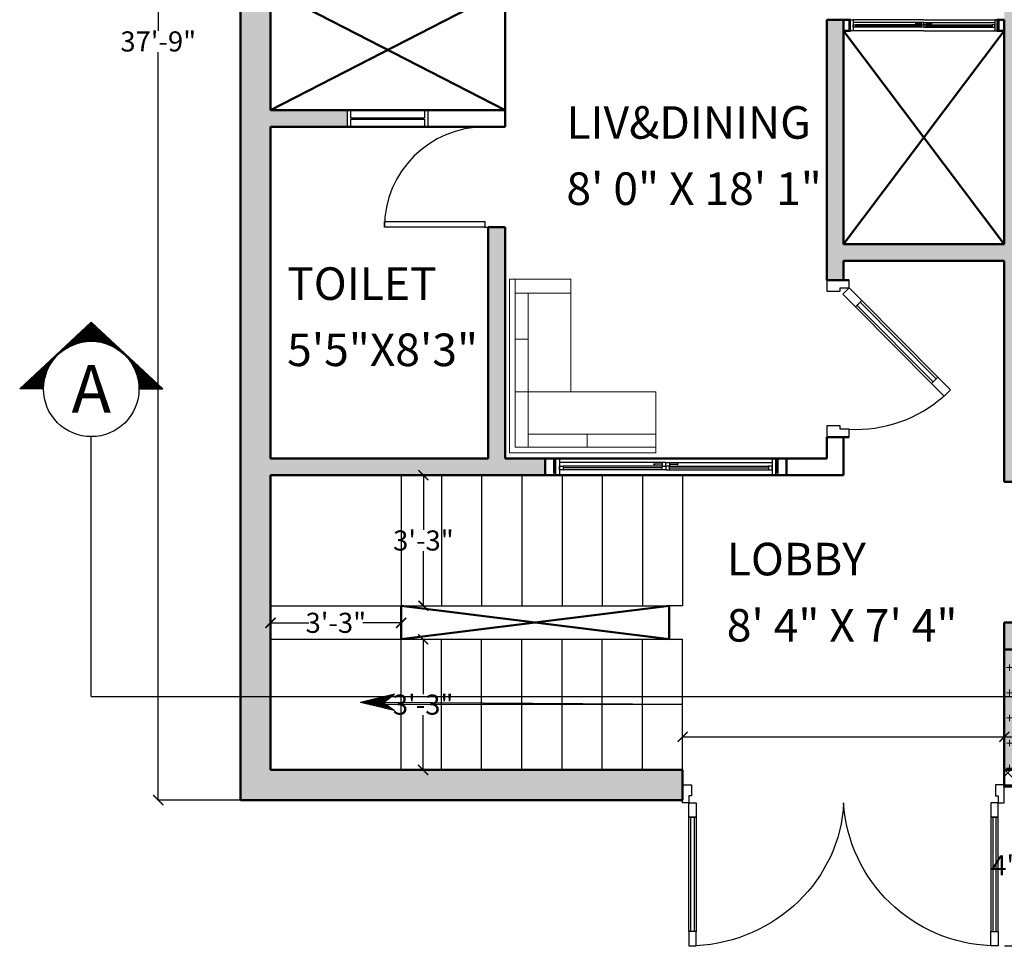
# Model space of a CAD drawing. Units: inches. Extents: x 2278 to 7495, y -71 to 1198.
# Tile 42 of 44: x 6921 to 7215, y 665 to 943. Entities that reach past the tile are written whole.
import ezdxf
from ezdxf.enums import TextEntityAlignment as Align

# ---------------------------------------------------------------- set-up
doc = ezdxf.new("R2010")
doc.units = ezdxf.units.IN
doc.header["$MEASUREMENT"] = 0
for name, color, linetype, lineweight in [('A-ANNO-DIMS', 2, 'Continuous', 18), ('A-ANNO-SYMB', 1, 'Continuous', 25), ('A-AREA-IDEN', 3, 'Continuous', 18), ('A-Door', 3, 'Continuous', 25), ('A-FLOR-PATT', 252, 'Continuous', 13), ('A-FLOR-STRS', 6, 'Continuous', 25), ('A-FURN', 8, 'Continuous', 18), ('A-Glaz', 4, 'Continuous', 25), ('A-Wall', 7, 'Continuous', 50), ('A-WALL-PATT', 8, 'Continuous', 18)]:
    doc.layers.add(name, color=color, linetype=linetype, lineweight=lineweight)
doc.styles.add('KH-TRUC', font='txt', dxfattribs={"height": 200})
doc.styles.get("Standard").update_dxf_attribs({"font": 'arial.ttf'})
doc.dimstyles.get("Standard").update_dxf_attribs({"dimtxt": 6, "dimasz": 3, "dimexe": 0.18, "dimexo": 0.0625, "dimgap": 0.09, "dimtad": 0, "dimtih": 1, "dimtoh": 1, "dimdec": 0, "dimzin": 0, "dimdsep": 46, "dimlunit": 3, "dimtxsty": 'Standard', "dimblk": 'ARCHTICK', "dimcen": 0.09, "dimadec": 0, "dimazin": 0, "dimtfac": 1, "dimtdec": 0, "dimtofl": 0, "dimtmove": 0, "dimatfit": 3, "dimfxl": 1, "dimtolj": 1, "dimtzin": 0, "dimarcsym": 0})

# ---------------------------------------------------------------- blocks, each defined once
blk = doc.blocks.new('*U5')
for p, q in [((0, 0), (0, -6)), ((30, 0), (30, -6))]:
    blk.add_line(p, q)
blk.add_lwpolyline([(0, 0), (0, 30), (1.75, 30), (1.75, 0)], close=True)
blk.add_arc((0, 0), 30, 0, 90)
blk = doc.blocks.new('A$C58286AE3')
for p, q in [((75, 820), (35, 820)), ((35, 820), (35, 180)), ((65, 820), (45, 820)), ((75, 180), (75, 820)), ((75, 180), (35, 180)), ((35, 180), (75, 180)), ((45, 180), (65, 180))]:
    blk.add_line(p, q)
blk.add_lwpolyline([(1725, 180), (1725, 820), (1765, 820), (1765, 180)], close=True)
blk.add_arc((1756.5, 42.1), 858.5, 92.1038, 176.1334)
blk.add_ellipse((70, 105), major_axis=(-772.1, 325.5), ratio=0.94084, start_param=-2.726592, end_param=-1.199193)
at = {"layer": 'A-Door'}
for p, q in [((35, 820), (35, 900)), ((35, 900), (75, 900)), ((75, 900), (75, 820)), ((75, 820), (35, 820)), ((35, 180), (35, 100)), ((75, 100), (75, 180)), ((35, 100), (0, 100)), ((0, 100), (0, 0)), ((35, 60), (35, 100)), ((35, 100), (75, 100)), ((50, 60), (35, 60)), ((50, 50), (50, 60)), ((50, 0), (50, 50)), ((0, 0), (50, 0))]:
    blk.add_line(p, q, dxfattribs=at)
for points in [[(1725, 900), (1725, 820), (1765, 820), (1765, 900)], [(1725, 100), (1725, 180), (1765, 180), (1765, 100)], [(1765, 100), (1800, 100), (1800, 0), (1750, 0), (1750, 50), (1750, 60), (1765, 60)]]:
    blk.add_lwpolyline(points, close=True, dxfattribs=at)
at = {"layer": 'A-Glaz'}
for p, q in [((45, 820), (45, 180)), ((65, 180), (65, 820))]:
    blk.add_line(p, q, dxfattribs=at)
blk.add_lwpolyline([(1735, 180), (1735, 820), (1755, 820), (1755, 180)], close=True, dxfattribs=at)
blk = doc.blocks.new('A$C1DF4181C')
blk.add_lwpolyline([(120, 128), (460.7, 466.1), (432.5, 494.5), (91.8, 156.4)], close=True)
blk.add_arc((72.4, 128.7), 593.3, 357.2313, 41.4937)
at = {"layer": 'A-Door'}
for points in [[(517.5, 522.4), (460.7, 466.1), (432.5, 494.5), (489.3, 550.8)], [(63.2, 71.6), (120, 128), (91.8, 156.4), (35, 100)], [(35, 100), (0, 100), (0, 0), (50, 0), (50, 50), (50, 60), (35, 60)], [(665, 100), (665, 60), (650, 60), (650, 50), (650, 0), (700, 0), (700, 100)]]:
    blk.add_lwpolyline(points, close=True, dxfattribs=at)
at = {"layer": 'A-Glaz'}
blk.add_lwpolyline([(112.9, 135.1), (453.6, 473.2), (439.5, 487.4), (98.8, 149.3)], close=True, dxfattribs=at)
at = {"layer": 'A-Wall'}
for p, q in [((0, 0), (0, 100)), ((0, 100), (0, 0)), ((700, 0), (700, 100)), ((700, 0), (700, 100))]:
    blk.add_line(p, q, dxfattribs=at)
blk = doc.blocks.new('_ArchTick')
at = {"color": 0, "linetype": 'ByBlock', "const_width": 0.15}
blk.add_lwpolyline([(-0.5, -0.5), (0.5, 0.5)], dxfattribs=at)
blk = doc.blocks.new('*D24')
at = {"layer": 'A-ANNO-DIMS', "color": 0, "lineweight": -2, "transparency": 16777216}
for p, q in [((7040.89, 807.47), (7041.94, 807.47)), ((7041.76, 807.47), (7041.76, 791.12)), ((7041.76, 768.47), (7041.76, 784.81)), ((7040.89, 768.47), (7041.94, 768.47))]:
    blk.add_line(p, q, dxfattribs=at)
at = {"layer": 'Defpoints', "color": 0, "transparency": 16777216}
for p in [(7040.83, 807.47), (7040.83, 768.47), (7041.76, 768.47)]:
    blk.add_point(p, dxfattribs=at)
at = {"layer": 'A-ANNO-DIMS', "color": 0, "lineweight": -2, "transparency": 16777216, "xscale": 3, "yscale": 3, "zscale": 3}
for p, rotation in [((7041.76, 807.47), 90), ((7041.76, 768.47), 270)]:
    blk.add_blockref('_ArchTick', p, dxfattribs=dict(at, rotation=rotation))
at = {"layer": 'A-ANNO-DIMS', "color": 0, "transparency": 16777216, "insert": (7041.76, 787.97), "char_height": 6, "attachment_point": 5}
blk.add_mtext('\\A1;3\'-3"', dxfattribs=at)
blk = doc.blocks.new('*D25')
at = {"layer": 'A-ANNO-DIMS', "color": 0, "lineweight": -2, "transparency": 16777216}
for p, q in [((6996.12, 763.4), (6996.12, 763.21)), ((6996.12, 763.39), (7007.55, 763.39)), ((7035.12, 763.39), (7023.68, 763.39)), ((7035.12, 763.4), (7035.12, 763.21))]:
    blk.add_line(p, q, dxfattribs=at)
at = {"layer": 'Defpoints', "color": 0, "transparency": 16777216}
for p in [(6996.12, 763.47), (7035.12, 763.47), (7035.12, 763.39)]:
    blk.add_point(p, dxfattribs=at)
at = {"layer": 'A-ANNO-DIMS', "color": 0, "lineweight": -2, "transparency": 16777216, "xscale": 3, "yscale": 3, "zscale": 3, "rotation": 180}
blk.add_blockref('_ArchTick', (6996.12, 763.39), dxfattribs=at)
at = {"layer": 'A-ANNO-DIMS', "color": 0, "lineweight": -2, "transparency": 16777216, "xscale": 3, "yscale": 3, "zscale": 3}
blk.add_blockref('_ArchTick', (7035.12, 763.39), dxfattribs=at)
at = {"layer": 'A-ANNO-DIMS', "color": 0, "transparency": 16777216, "insert": (7015.62, 763.39), "char_height": 6, "attachment_point": 5}
blk.add_mtext('\\A1;3\'-3"', dxfattribs=at)
blk = doc.blocks.new('*D26')
at = {"layer": 'A-ANNO-DIMS', "color": 0, "lineweight": -2, "transparency": 16777216}
for p, q in [((7040.86, 758.47), (7041.85, 758.47)), ((7041.67, 758.47), (7041.67, 742.12)), ((7041.67, 719.47), (7041.67, 735.81)), ((7040.86, 719.47), (7041.85, 719.47))]:
    blk.add_line(p, q, dxfattribs=at)
at = {"layer": 'Defpoints', "color": 0, "transparency": 16777216}
for p in [(7040.8, 758.47), (7040.8, 719.47), (7041.67, 719.47)]:
    blk.add_point(p, dxfattribs=at)
at = {"layer": 'A-ANNO-DIMS', "color": 0, "lineweight": -2, "transparency": 16777216, "xscale": 3, "yscale": 3, "zscale": 3}
for p, rotation in [((7041.67, 758.47), 90), ((7041.67, 719.47), 270)]:
    blk.add_blockref('_ArchTick', p, dxfattribs=dict(at, rotation=rotation))
at = {"layer": 'A-ANNO-DIMS', "color": 0, "transparency": 16777216, "insert": (7041.67, 738.97), "char_height": 6, "attachment_point": 5}
blk.add_mtext('\\A1;3\'-3"', dxfattribs=at)
blk = doc.blocks.new('*D27')
at = {"layer": 'A-ANNO-DIMS', "color": 0, "lineweight": -2, "transparency": 16777216}
for p, q in [((6987.05, 1163.47), (6962.44, 1163.47)), ((6962.62, 1163.47), (6962.62, 940.12)), ((6962.62, 710.47), (6962.62, 933.81)), ((6987.05, 710.47), (6962.44, 710.47))]:
    blk.add_line(p, q, dxfattribs=at)
at = {"layer": 'Defpoints', "color": 0, "transparency": 16777216}
for p in [(6987.12, 1163.47), (6962.62, 710.47), (6987.12, 710.47)]:
    blk.add_point(p, dxfattribs=at)
at = {"layer": 'A-ANNO-DIMS', "color": 0, "lineweight": -2, "transparency": 16777216, "xscale": 3, "yscale": 3, "zscale": 3}
for p, rotation in [((6962.62, 1163.47), 90), ((6962.62, 710.47), 270)]:
    blk.add_blockref('_ArchTick', p, dxfattribs=dict(at, rotation=rotation))
at = {"layer": 'A-ANNO-DIMS', "color": 0, "transparency": 16777216, "insert": (6962.62, 936.97), "char_height": 6, "attachment_point": 5}
blk.add_mtext('\\A1;37\'-9"', dxfattribs=at)
blk = doc.blocks.new('*X31')
at = {"color": 0}
for p, q in [((19.68, 20.47), (19.71, 20.51)), ((19.68, 20.38), (19.76, 20.46)), ((19.68, 20.29), (19.8, 20.42)), ((19.68, 20.21), (19.84, 20.37)), ((19.68, 20.12), (19.88, 20.33)), ((19.68, 20.03), (19.93, 20.28)), ((19.68, 19.94), (19.97, 20.23)), ((19.68, 19.85), (20.01, 20.19)), ((19.68, 19.76), (20.05, 20.14)), ((19.68, 19.68), (20.1, 20.1)), ((19.68, 19.59), (20.14, 20.05)), ((19.68, 19.5), (20.18, 20.01)), ((19.68, 19.41), (20.22, 19.96)), ((19.68, 19.32), (20.27, 19.91)), ((19.68, 19.23), (20.31, 19.87)), ((19.68, 19.15), (20.35, 19.82)), ((19.68, 19.06), (20.4, 19.78)), ((19.68, 18.97), (20.44, 19.73)), ((19.68, 18.88), (20.48, 19.69)), ((19.68, 18.79), (20.52, 19.64)), ((19.68, 18.7), (20.57, 19.59)), ((19.68, 18.62), (20.61, 19.55)), ((19.68, 18.53), (20.65, 19.5)), ((19.68, 18.44), (20.69, 19.46)), ((19.68, 18.35), (20.74, 19.41)), ((19.68, 18.26), (20.78, 19.37)), ((19.68, 18.17), (20.82, 19.32)), ((19.68, 18.08), (20.86, 19.27)), ((19.73, 18.05), (20.91, 19.23)), ((19.81, 18.05), (20.95, 19.18)), ((19.9, 18.04), (20.99, 19.14)), ((19.98, 18.04), (21.04, 19.09)), ((20.06, 18.03), (21.08, 19.05)), ((20.15, 18.03), (21.12, 19)), ((20.23, 18.02), (21.16, 18.95)), ((20.31, 18.01), (21.21, 18.91)), ((20.38, 18), (21.25, 18.86)), ((20.46, 17.99), (21.29, 18.82)), ((20.54, 17.97), (21.33, 18.77)), ((20.61, 17.96), (21.38, 18.73)), ((20.68, 17.94), (21.42, 18.68)), ((20.76, 17.93), (21.46, 18.63)), ((20.83, 17.91), (21.5, 18.59)), ((20.9, 17.9), (21.55, 18.54)), ((20.97, 17.88), (21.59, 18.5)), ((21.04, 17.86), (21.63, 18.45)), ((21.11, 17.84), (21.68, 18.41)), ((21.18, 17.82), (21.72, 18.36)), ((21.24, 17.8), (21.76, 18.31)), ((21.31, 17.77), (21.8, 18.27)), ((21.37, 17.75), (21.85, 18.22)), ((21.44, 17.73), (21.89, 18.18)), ((21.5, 17.7), (21.93, 18.13)), ((21.57, 17.68), (21.97, 18.08)), ((21.63, 17.65), (22.02, 18.04)), ((21.69, 17.62), (22.06, 17.99)), ((21.75, 17.6), (22.1, 17.95)), ((21.81, 17.57), (22.14, 17.9)), ((21.87, 17.54), (22.19, 17.86)), ((21.93, 17.51), (22.23, 17.81)), ((21.99, 17.48), (22.27, 17.76)), ((22.05, 17.45), (22.32, 17.72)), ((22.1, 17.42), (22.36, 17.67)), ((22.16, 17.39), (22.4, 17.63)), ((22.22, 17.35), (22.44, 17.58)), ((22.27, 17.32), (22.49, 17.54)), ((22.33, 17.29), (22.53, 17.49)), ((22.38, 17.25), (22.57, 17.44)), ((22.43, 17.22), (22.61, 17.4)), ((22.49, 17.18), (22.66, 17.35)), ((22.54, 17.15), (22.7, 17.31)), ((22.59, 17.11), (22.74, 17.26)), ((22.64, 17.07), (22.78, 17.22)), ((22.69, 17.04), (22.83, 17.17)), ((22.74, 17), (22.87, 17.12)), ((22.79, 16.96), (22.91, 17.08)), ((22.84, 16.92), (22.96, 17.03)), ((22.89, 16.88), (23, 16.99)), ((22.94, 16.84), (23.04, 16.94)), ((22.98, 16.8), (23.08, 16.9)), ((23.03, 16.75), (23.13, 16.85)), ((23.08, 16.71), (23.17, 16.8)), ((23.12, 16.67), (23.21, 16.76)), ((23.17, 16.63), (23.25, 16.71)), ((23.21, 16.58), (23.3, 16.67)), ((23.26, 16.54), (23.34, 16.62)), ((23.3, 16.49), (23.38, 16.58)), ((23.34, 16.45), (23.42, 16.53)), ((23.38, 16.4), (23.47, 16.48)), ((23.43, 16.35), (23.51, 16.44)), ((23.47, 16.31), (23.55, 16.39)), ((23.51, 16.26), (23.6, 16.35)), ((23.55, 16.21), (23.64, 16.3)), ((23.59, 16.16), (23.68, 16.26)), ((23.63, 16.11), (23.72, 16.21)), ((23.66, 16.06), (23.77, 16.16)), ((23.7, 16.01), (23.81, 16.12)), ((23.74, 15.96), (23.85, 16.07)), ((23.78, 15.91), (23.89, 16.03)), ((23.81, 15.86), (23.94, 15.98)), ((23.85, 15.8), (23.98, 15.94)), ((23.88, 15.75), (24.02, 15.89)), ((23.92, 15.7), (24.06, 15.84)), ((23.95, 15.64), (24.11, 15.8)), ((23.98, 15.59), (24.15, 15.75)), ((24.02, 15.53), (24.19, 15.71)), ((24.05, 15.47), (24.24, 15.66)), ((24.08, 15.42), (24.28, 15.62)), ((24.11, 15.36), (24.32, 15.57)), ((24.14, 15.3), (24.36, 15.52)), ((24.17, 15.24), (24.41, 15.48)), ((24.2, 15.18), (24.45, 15.43)), ((24.23, 15.12), (24.49, 15.39)), ((24.25, 15.06), (24.53, 15.34)), ((24.28, 15), (24.58, 15.3)), ((24.31, 14.94), (24.62, 15.25)), ((24.33, 14.87), (24.66, 15.2)), ((24.36, 14.81), (24.7, 15.16)), ((24.38, 14.74), (24.75, 15.11)), ((24.4, 14.68), (24.79, 15.07)), ((24.42, 14.61), (24.83, 15.02)), ((24.45, 14.55), (24.88, 14.98)), ((24.47, 14.48), (24.92, 14.93)), ((24.49, 14.41), (24.96, 14.88)), ((24.51, 14.34), (25, 14.84)), ((24.52, 14.27), (25.05, 14.79)), ((24.54, 14.2), (25.09, 14.75)), ((24.56, 14.13), (25.13, 14.7)), ((24.57, 14.06), (25.17, 14.66)), ((24.59, 13.98), (25.22, 14.61)), ((24.6, 13.91), (25.26, 14.56)), ((24.61, 13.83), (25.3, 14.52)), ((24.63, 13.75), (25.35, 14.47)), ((24.44, 11.54), (26.33, 13.42)), ((24.48, 11.66), (26.28, 13.47)), ((24.51, 11.79), (26.24, 13.51)), ((24.54, 11.9), (26.2, 13.56)), ((24.57, 12.02), (26.16, 13.6)), ((24.59, 12.13), (26.11, 13.65)), ((24.61, 12.24), (26.07, 13.7)), ((24.63, 12.34), (26.03, 13.74)), ((24.64, 13.68), (25.39, 14.43)), ((24.64, 12.44), (25.99, 13.79)), ((24.65, 13.6), (25.43, 14.38)), ((24.65, 13.52), (25.47, 14.34)), ((24.65, 12.54), (25.94, 13.83)), ((24.66, 13.44), (25.52, 14.29)), ((24.66, 12.64), (25.9, 13.88)), ((24.67, 13.35), (25.56, 14.24)), ((24.67, 13.27), (25.6, 14.2)), ((24.67, 13.18), (25.64, 14.15)), ((24.67, 12.92), (25.77, 14.02)), ((24.67, 12.83), (25.81, 13.97)), ((24.67, 12.73), (25.86, 13.92)), ((24.68, 13.1), (25.69, 14.11)), ((24.68, 13.01), (25.73, 14.06)), ((23.72, 10.11), (26.67, 13.06)), ((23.91, 10.38), (26.63, 13.1)), ((24.04, 10.6), (26.58, 13.15)), ((24.14, 10.79), (26.54, 13.19)), ((24.22, 10.96), (26.5, 13.24)), ((24.29, 11.12), (26.45, 13.28)), ((24.35, 11.27), (26.41, 13.33)), ((24.4, 11.41), (26.37, 13.38)), ((19.68, 5.98), (25.68, 11.98)), ((19.68, 5.89), (24.44, 10.65)), ((19.68, 5.8), (23.2, 9.32)), ((19.68, 6.06), (22.61, 9)), ((19.68, 6.15), (22.34, 8.81)), ((19.68, 6.24), (22.12, 8.69)), ((19.68, 6.33), (21.93, 8.58)), ((19.68, 6.42), (21.76, 8.5)), ((19.68, 6.51), (21.6, 8.43)), ((19.68, 6.59), (21.46, 8.37)), ((19.68, 6.68), (21.32, 8.32)), ((19.68, 6.77), (21.19, 8.28)), ((19.68, 6.86), (21.06, 8.24)), ((19.68, 6.95), (20.94, 8.21)), ((19.68, 7.04), (20.82, 8.18)), ((19.68, 7.12), (20.71, 8.15)), ((19.68, 7.21), (20.6, 8.13)), ((19.68, 7.3), (20.49, 8.11)), ((19.68, 7.39), (20.38, 8.1)), ((19.68, 7.48), (20.28, 8.08)), ((19.68, 7.57), (20.18, 8.07)), ((19.68, 7.74), (19.99, 8.06)), ((19.68, 7.66), (20.08, 8.06)), ((19.68, 8.01), (19.71, 8.05)), ((19.68, 7.92), (19.8, 8.05)), ((19.68, 7.83), (19.9, 8.05)), ((19.68, 5.71), (21.96, 8)), ((19.68, 5.62), (20.73, 6.67))]:
    blk.add_line(p, q, dxfattribs=at)
blk = doc.blocks.new('A$C695C76AC')
for p, q in [((5.36, 5), (12.86, 12)), ((20.36, 5), (12.86, 12)), ((7.86, 5), (5.36, 5)), ((17.86, 5), (20.36, 5))]:
    blk.add_line(p, q)
blk.add_circle((12.86, 5), 5)
at = {"rotation": 90}
blk.add_blockref('*X31', (25.9, -14.68), dxfattribs=at)
at = {"style": 'KH-TRUC'}
blk.add_attdef('KH-MC', text='', height=5, dxfattribs=at).set_placement((12.86, 5), align=Align.MIDDLE_CENTER)
blk = doc.blocks.new('*D55')
at = {"layer": 'A-ANNO-DIMS', "color": 0, "lineweight": -2, "transparency": 16777216}
for p, q in [((7119.12, 715.03), (7119.12, 729.55)), ((7119.12, 729.37), (7215.12, 729.37)), ((7215.12, 715.03), (7215.12, 729.55)), ((7215.12, 729.37), (7218.12, 729.37))]:
    blk.add_line(p, q, dxfattribs=at)
at = {"layer": 'Defpoints', "color": 0, "transparency": 16777216}
for p in [(7215.12, 729.37), (7119.12, 714.97), (7215.12, 714.97)]:
    blk.add_point(p, dxfattribs=at)
at = {"layer": 'A-ANNO-DIMS', "color": 0, "lineweight": -2, "transparency": 16777216, "xscale": 3, "yscale": 3, "zscale": 3, "rotation": 180}
blk.add_blockref('_ArchTick', (7119.12, 729.37), dxfattribs=at)
at = {"layer": 'A-ANNO-DIMS', "color": 0, "lineweight": -2, "transparency": 16777216, "xscale": 3, "yscale": 3, "zscale": 3}
blk.add_blockref('_ArchTick', (7215.12, 729.37), dxfattribs=at)
at = {"layer": 'A-ANNO-DIMS', "color": 0, "transparency": 16777216, "insert": (7285.95, 729.37), "char_height": 6, "attachment_point": 5}
blk.add_mtext('\\A1;MAIN ENTRANCE DOOR 8\'-0" TYP.', dxfattribs=at)
blk = doc.blocks.new('*D56')
at = {"layer": 'A-ANNO-DIMS', "color": 0, "lineweight": -2, "transparency": 16777216}
for p, q in [((7215.18, 714.97), (7229.7, 714.97)), ((7229.52, 714.97), (7229.52, 694.12)), ((7229.52, 666.97), (7229.52, 687.81)), ((7215.18, 666.97), (7229.7, 666.97))]:
    blk.add_line(p, q, dxfattribs=at)
at = {"layer": 'Defpoints', "color": 0, "transparency": 16777216}
for p in [(7215.12, 714.97), (7215.12, 666.97), (7229.52, 666.97)]:
    blk.add_point(p, dxfattribs=at)
at = {"layer": 'A-ANNO-DIMS', "color": 0, "lineweight": -2, "transparency": 16777216, "xscale": 3, "yscale": 3, "zscale": 3}
for p, rotation in [((7229.52, 714.97), 90), ((7229.52, 666.97), 270)]:
    blk.add_blockref('_ArchTick', p, dxfattribs=dict(at, rotation=rotation))
at = {"layer": 'A-ANNO-DIMS', "color": 0, "transparency": 16777216, "insert": (7229.52, 690.97), "char_height": 6, "attachment_point": 5}
blk.add_mtext('\\A1;4\'-0" TYP.', dxfattribs=at)

msp = doc.modelspace()

# ---------------------------------------------------------------- hatches: boundary and pattern name
at = {"layer": 'A-FLOR-PATT'}
h = msp.add_hatch(dxfattribs=at)
h.set_pattern_fill('ANSI31', color=256)
h.set_pattern_definition([(45, (4673.24527, 0), (-0.0883883476, 0.0883883476), [])])
h.paths.add_polyline_path([(7029.84, 739.64), (7033.16, 742.09), (7022.93, 739.64), (7033.16, 737.18)])
at = {"layer": 'A-WALL-PATT'}
h = msp.add_hatch(dxfattribs=at)
h.set_pattern_fill('ANSI36', color=256, scale=30)
h.set_pattern_definition([(45, (4673.2453, 0), (1.988738, 7.2920387), [9.375, -1.875, 0, -1.875])])
h.paths.add_polyline_path([(7016.37, 957.47), (6996.12, 957.47), (6996.12, 1029.47), (7025.12, 1029.47), (7025.12, 1034.47), (6996.12, 1034.47), (6996.12, 1154.47), (7013.12, 1154.47), (7013.12, 1163.47), (6987.12, 1163.47), (6987.12, 710.47), (7119.12, 710.47), (7119.12, 719.47), (6996.12, 719.47), (6996.12, 807.47), (7078.12, 807.47), (7078.12, 812.47), (7066.12, 812.47), (7066.12, 881.47), (7061.12, 881.47), (7061.12, 812.47), (6996.12, 812.47), (6996.12, 911.47), (7019.12, 911.47), (7019.12, 916.47), (6996.12, 916.47), (6996.12, 952.47), (7016.37, 952.47)])
h.paths.add_polyline_path([(7125.12, 1163.47), (7085.12, 1163.47), (7085.12, 1154.47), (7102.12, 1154.47), (7102.12, 1034.47), (7102.12, 1029.47), (7107.12, 1029.47), (7107.12, 1154.47), (7125.12, 1154.47)])
h.paths.add_polyline_path([(7232.12, 1163.47), (7197.12, 1163.47), (7197.12, 1154.47), (7215.12, 1154.47), (7215.12, 1034.47), (7149.12, 1034.47), (7149.12, 1029.47), (7215.12, 1029.47), (7215.12, 943.47), (7215.12, 940.13), (7215.12, 876.47), (7167.12, 876.47), (7167.12, 943.47), (7162.12, 943.47), (7162.12, 871.47), (7162.12, 865.74), (7167.12, 865.74), (7167.12, 871.47), (7215.12, 871.47), (7215.12, 805.47), (7220.12, 805.47), (7220.12, 1077.47), (7232.12, 1077.47), (7232.12, 1082.47), (7220.12, 1082.47), (7220.12, 1154.47), (7232.12, 1154.47)])
h.paths.add_polyline_path([(7390.12, 937.97), (7381.12, 937.97), (7381.12, 911.47), (7268.12, 911.47), (7268.12, 906.47), (7381.12, 906.47), (7381.12, 869.47), (7390.12, 869.47)])
h.paths.add_polyline_path([(7390.12, 1163.47), (7363.12, 1163.47), (7363.12, 1154.47), (7381.12, 1154.47), (7381.12, 1041.47), (7268.12, 1041.47), (7268.12, 1036.47), (7381.12, 1036.47), (7381.12, 1009.97), (7390.12, 1009.97)])
h.paths.add_polyline_path([(7291.12, 1163.47), (7256.12, 1163.47), (7256.12, 1154.47), (7268.12, 1154.47), (7268.12, 1082.47), (7262.12, 1082.47), (7262.12, 1077.47), (7273.12, 1077.47), (7273.12, 1154.47), (7291.12, 1154.47)])
h.paths.add_polyline_path([(7390.12, 797.47), (7381.12, 797.47), (7381.12, 760.47), (7336.62, 760.47), (7336.62, 755.47), (7390.12, 755.47)])
h.paths.add_polyline_path([(7264.62, 760.47), (7220.12, 760.47), (7220.12, 763.47), (7215.12, 763.47), (7215.12, 755.47), (7264.62, 755.47)])
h = msp.add_hatch(dxfattribs=at)
h.set_pattern_fill('ANSI37', color=256, scale=30)
h.set_pattern_definition([(45, (4673.2453, 0), (-2.6516504, 2.6516504), []), (135, (4673.2453, 0), (-2.6516504, -2.6516504), [])])
h.paths.add_polyline_path([(7390.12, 755.47), (7381.12, 755.47), (7381.12, 719.47), (7215.12, 719.47), (7215.12, 714.47), (7390.12, 714.47)])
at = {"layer": 'A-WALL-PATT', "transparency": 33554562}
h = msp.add_hatch(color=256, dxfattribs=at)
h.dxf.hatch_style = 1
h.paths.add_polyline_path([(7381.12, 755.47), (7215.12, 755.47), (7215.12, 719.47), (7381.12, 719.47)])
h = msp.add_hatch(dxfattribs=at)
h.set_pattern_fill('CROSS', color=256, scale=15)
h.set_pattern_definition([(0, (4673.2453, 0), (3.75, 3.75), [1.875, -5.625]), (90, (4674.1828, -0.9375), (-3.75, 3.75), [1.875, -5.625])])
h.paths.add_polyline_path([(7381.12, 755.47), (7215.12, 755.47), (7215.12, 719.47), (7381.12, 719.47)])

# ---------------------------------------------------------------- linework, layer by layer
at = {"layer": 'A-ANNO-SYMB'}
for q in [(6942.63, 818.97), (7473.67, 741.41)]:
    msp.add_line((6942.63, 741.41), q, dxfattribs=at)
at = {"layer": 'A-FLOR-STRS'}
for p, q in [((7035.12, 807.47), (7035.12, 768.47)), ((7047.12, 807.47), (7047.12, 768.47)), ((7059.12, 807.47), (7059.12, 768.47)), ((7071.12, 807.47), (7071.12, 768.47)), ((7083.12, 807.47), (7083.12, 768.47)), ((7095.12, 807.47), (7095.12, 768.47)), ((7107.12, 807.47), (7107.12, 768.47)), ((7119.12, 807.47), (7119.12, 768.47)), ((6996.12, 768.47), (7115.12, 768.47)), ((7119.12, 768.47), (7115.12, 768.47)), ((6996.12, 758.47), (7119.12, 758.47)), ((7035.12, 719.47), (7035.12, 758.47)), ((7047.12, 719.47), (7047.12, 758.47)), ((7059.12, 719.47), (7059.12, 758.47)), ((7071.12, 719.47), (7071.12, 758.47)), ((7083.12, 719.47), (7083.12, 758.47)), ((7095.12, 719.47), (7095.12, 758.47)), ((7107.12, 719.47), (7107.12, 758.47)), ((7119.12, 719.47), (7119.12, 758.47)), ((7033.16, 742.09), (7022.93, 739.64)), ((7029.84, 739.64), (7033.16, 742.09)), ((7033.16, 737.18), (7022.93, 739.64)), ((7119.12, 738.97), (7029.84, 739.64)), ((7029.84, 739.64), (7033.16, 737.18)), ((7119.12, 738.97), (7030.58, 738.97))]:
    msp.add_line(p, q, dxfattribs=at)
at = {"layer": 'A-FURN'}
for p, q in [((7067.46, 814.1), (7067.46, 866.04)), ((7085.7, 866.04), (7067.46, 866.04)), ((7069.15, 815.79), (7069.15, 866.04)), ((7085.7, 832.34), (7085.7, 866.04)), ((7085.7, 861.82), (7069.15, 861.82)), ((7073.03, 815.79), (7073.03, 861.82)), ((7073.03, 848.05), (7069.15, 848.05)), ((7111.07, 832.34), (7069.15, 832.34)), ((7111.07, 814.1), (7111.07, 832.34)), ((7073.03, 819.67), (7111.07, 819.67)), ((7090.59, 815.79), (7090.59, 819.67)), ((7111.07, 814.1), (7067.46, 814.1)), ((7069.15, 815.79), (7111.07, 815.79))]:
    msp.add_line(p, q, dxfattribs=at)
at = {"layer": 'A-Glaz'}
for p, q in [((7191.12, 943.47), (7169.97, 943.47)), ((7191.12, 943.47), (7212.26, 943.47)), ((7191.12, 942.66), (7169.97, 942.66)), ((7190.39, 941.94), (7170.69, 941.94)), ((7190.39, 941.58), (7170.69, 941.58)), ((7190.39, 941.22), (7170.69, 941.22)), ((7190.39, 942.3), (7188.84, 942.3)), ((7191.12, 942.66), (7212.26, 942.66)), ((7191.84, 942.3), (7193.39, 942.3)), ((7191.84, 941.94), (7211.54, 941.94)), ((7191.84, 941.58), (7211.54, 941.58)), ((7191.84, 941.22), (7211.54, 941.22)), ((7191.12, 940.13), (7169.97, 940.13)), ((7191.12, 940.13), (7212.26, 940.13)), ((7019.12, 916.47), (7043.12, 916.47)), ((7019.12, 911.47), (7019.12, 916.47)), ((7020.12, 914.17), (7020.12, 916.47)), ((7020.12, 914.17), (7042.12, 914.17)), ((7042.12, 916.47), (7042.12, 914.17)), ((7043.12, 916.47), (7043.12, 911.47)), ((7043.12, 911.47), (7019.12, 911.47)), ((7020.12, 911.47), (7020.12, 913.77)), ((7020.12, 913.77), (7042.12, 913.77)), ((7042.12, 913.77), (7042.12, 911.47)), ((7114.12, 812.47), (7082.39, 812.47)), ((7114.12, 811.26), (7082.39, 811.26)), ((7114.12, 812.47), (7145.84, 812.47)), ((7114.12, 811.26), (7145.84, 811.26)), ((7113.03, 810.18), (7083.48, 810.18)), ((7113.03, 809.64), (7083.48, 809.64)), ((7113.03, 809.09), (7083.48, 809.09)), ((7113.03, 810.72), (7110.7, 810.72)), ((7115.2, 810.72), (7117.53, 810.72)), ((7115.2, 810.18), (7144.75, 810.18)), ((7115.2, 809.64), (7144.75, 809.64)), ((7115.2, 809.09), (7144.75, 809.09)), ((7114.12, 807.47), (7082.39, 807.47)), ((7114.12, 807.47), (7145.84, 807.47))]:
    msp.add_line(p, q, dxfattribs=at)
for points in [[(7169.97, 940.13), (7169.24, 940.13), (7169.24, 943.47), (7169.97, 943.47)], [(7212.26, 940.13), (7212.99, 940.13), (7212.99, 943.47), (7212.26, 943.47)], [(7170.69, 941.22), (7169.97, 941.22), (7169.97, 941.94), (7170.69, 941.94)], [(7188.65, 942.3), (7188.84, 942.41), (7188.84, 942.19)], [(7190.39, 941.94), (7191.12, 941.94), (7191.12, 942.66), (7190.39, 942.66)], [(7191.12, 941.22), (7190.39, 941.22), (7190.39, 941.94), (7191.12, 941.94)], [(7191.84, 941.94), (7191.12, 941.94), (7191.12, 942.66), (7191.84, 942.66)], [(7191.12, 941.22), (7191.84, 941.22), (7191.84, 941.94), (7191.12, 941.94)], [(7193.58, 942.3), (7193.39, 942.41), (7193.39, 942.19)], [(7211.54, 941.22), (7212.26, 941.22), (7212.26, 941.94), (7211.54, 941.94)], [(7082.39, 807.47), (7081.31, 807.47), (7081.31, 812.47), (7082.39, 812.47)], [(7113.03, 810.18), (7114.12, 810.18), (7114.12, 811.26), (7113.03, 811.26)], [(7115.2, 810.18), (7114.12, 810.18), (7114.12, 811.26), (7115.2, 811.26)], [(7145.84, 807.47), (7146.92, 807.47), (7146.92, 812.47), (7145.84, 812.47)], [(7083.48, 809.09), (7082.39, 809.09), (7082.39, 810.18), (7083.48, 810.18)], [(7110.42, 810.72), (7110.7, 810.88), (7110.7, 810.56)], [(7114.12, 809.09), (7113.03, 809.09), (7113.03, 810.18), (7114.12, 810.18)], [(7114.12, 809.09), (7115.2, 809.09), (7115.2, 810.18), (7114.12, 810.18)], [(7117.81, 810.72), (7117.53, 810.88), (7117.53, 810.56)], [(7144.75, 809.09), (7145.84, 809.09), (7145.84, 810.18), (7144.75, 810.18)]]:
    msp.add_lwpolyline(points, close=True, dxfattribs=at)
at = {"layer": 'A-Wall'}
for p, q in [((6987.12, 1163.47), (6987.12, 710.47)), ((7066.12, 1029.47), (7066.12, 911.47)), ((6996.12, 952.47), (6996.12, 916.47)), ((7066.12, 916.47), (6996.12, 952.47)), ((6996.12, 916.47), (7066.12, 952.47)), ((7162.12, 943.47), (7162.12, 871.47)), ((7167.12, 943.47), (7162.12, 943.47)), ((7167.12, 943.47), (7167.12, 876.47)), ((7167.12, 940.13), (7167.12, 943.47)), ((7169.24, 943.47), (7167.12, 943.47)), ((7168.88, 943.39), (7168.88, 940.49)), ((7212.99, 943.47), (7215.12, 943.47)), ((7213.35, 943.39), (7213.35, 940.49)), ((7215.12, 943.47), (7215.12, 876.47)), ((7215.12, 940.13), (7215.12, 943.47)), ((7169.24, 940.13), (7167.12, 940.13)), ((7167.12, 876.47), (7215.12, 940.13)), ((7215.12, 876.47), (7167.12, 940.13)), ((7212.99, 940.13), (7215.12, 940.13)), ((6996.12, 916.47), (7066.12, 916.47)), ((6996.12, 911.47), (6996.12, 812.47)), ((6996.12, 911.47), (7066.12, 911.47)), ((7061.12, 881.47), (7061.12, 812.47)), ((7061.12, 881.47), (7066.12, 881.47)), ((7066.12, 881.47), (7066.12, 812.47)), ((7167.12, 876.47), (7215.12, 876.47)), ((7162.12, 871.47), (7162.12, 865.74)), ((7167.12, 871.47), (7215.12, 871.47)), ((7167.12, 865.74), (7167.12, 871.47)), ((7215.12, 871.47), (7215.12, 805.47)), ((7162.12, 865.74), (7167.12, 865.74)), ((7162.12, 812.47), (7162.12, 818.82)), ((7162.12, 818.82), (7167.08, 818.82)), ((7167.08, 818.82), (7167.12, 812.47)), ((6996.12, 812.47), (7061.12, 812.47)), ((7066.12, 812.47), (7162.12, 812.47)), ((7078.12, 807.47), (7078.12, 812.47)), ((7081.31, 812.47), (7078.12, 812.47)), ((7080.77, 812.35), (7080.77, 808.01)), ((7146.92, 812.47), (7150.12, 812.47)), ((7147.46, 812.35), (7147.46, 808.01)), ((7150.12, 807.47), (7150.12, 812.47)), ((7167.12, 812.47), (7167.12, 807.47)), ((6996.12, 807.47), (6996.12, 719.47)), ((6996.12, 807.47), (7167.12, 807.47)), ((7081.31, 807.47), (7078.12, 807.47)), ((7146.92, 807.47), (7150.12, 807.47)), ((7220.12, 805.47), (7215.12, 805.47)), ((7035.12, 758.47), (7035.12, 768.47)), ((7035.12, 758.47), (7115.12, 768.47)), ((7115.12, 758.47), (7035.12, 768.47)), ((7115.12, 768.47), (7115.12, 758.47)), ((7215.12, 763.47), (7215.12, 755.47)), ((7220.12, 763.47), (7215.12, 763.47)), ((7215.12, 755.47), (7390.12, 755.47)), ((7215.12, 755.47), (7215.12, 719.47)), ((6996.12, 719.47), (7119.12, 719.47)), ((7119.12, 710.47), (7119.12, 719.47)), ((7215.12, 719.47), (7215.12, 714.47)), ((7215.12, 719.47), (7381.12, 719.47)), ((7215.12, 714.47), (7390.12, 714.47)), ((6987.12, 710.47), (7119.12, 710.47))]:
    msp.add_line(p, q, dxfattribs=at)

# ---------------------------------------------------------------- block references
at = {"layer": 'A-ANNO-SYMB'}
ref = msp.add_blockref('A$C695C76AC', (6906.01, 818.97), dxfattribs=dict(at, xscale=2.847836231539501, yscale=2.847836231539501, zscale=2.847836231539501))
ref.add_attrib('KH-MC', 'A', dxfattribs={"layer": '0', "color": 3, "height": 14.24, "style": 'KH-TRUC'}).set_placement((6942.63, 833.21), align=Align.MIDDLE_CENTER)
at = {"layer": 'A-Door', "rotation": 89.99999999999999}
msp.add_blockref('*U5', (7060.12, 881.47), dxfattribs=at)
at = {"layer": 'A-Door'}
for name, p, xscale, yscale, zscale, rotation in [('A$C1DF4181C', (7162.12, 865.74), 0.0670393380383952, 0.0670393380383952, 0.0670393380383952, 270), ('A$C58286AE3', (7119.12, 714.97), -0.0533333333333331, 0.0533333333333331, 0.0533333333333331, 180)]:
    msp.add_blockref(name, p, dxfattribs=dict(at, xscale=xscale, yscale=yscale, zscale=zscale, rotation=rotation))

# ---------------------------------------------------------------- texts
at = {"layer": 'A-AREA-IDEN'}
for s, height, p in [('LIV&DINING', 9.72, (7084.43, 907.92)), ('8\' 0" X 18\' 1"', 9.7203, (7084.43, 888.15)), ('TOILET', 9.72, (7001.08, 859.81)), ('5\'5"X8\'3"', 9.72, (7001.08, 840.04)), ('LOBBY', 9.72, (7132.29, 777.56)), ('8\' 4" X 7\' 4"', 9.7203, (7132.29, 757.78))]:
    msp.add_text(s, height=height, dxfattribs=at).set_placement(p)

# ---------------------------------------------------------------- dimensions: what is measured, and where the dimension line sits
at = {"layer": 'A-ANNO-DIMS'}
for base, p1, p2, picture, middle in [((6962.62, 710.47), (6987.12, 1163.47), (6987.12, 710.47), '*D27', (6962.62, 936.97)), ((7041.76, 768.47), (7040.83, 807.47), (7040.83, 768.47), '*D24', (7041.76, 787.97)), ((7041.67, 719.47), (7040.8, 758.47), (7040.8, 719.47), '*D26', (7041.67, 738.97))]:
    dim = msp.add_linear_dim(base=base, p1=p1, p2=p2, angle=90, dimstyle='Standard', override={"dimclrd": 0, "dimclre": 0, "dimclrt": 0}, dxfattribs=at)
    dim.commit()
    dim.dimension.update_dxf_attribs({"geometry": picture, "text_midpoint": middle})
dim = msp.add_linear_dim(base=(7035.12, 763.39), p1=(6996.12, 763.47), p2=(7035.12, 763.47), dimstyle='Standard', override={"dimclrd": 0, "dimclre": 0, "dimclrt": 0}, dxfattribs=at)
dim.commit()
dim.dimension.update_dxf_attribs({"geometry": '*D25', "text_midpoint": (7015.62, 763.39)})
dim = msp.add_linear_dim(base=(7215.12, 729.37), p1=(7119.12, 714.97), p2=(7215.12, 714.97), text='MAIN ENTRANCE DOOR <> TYP.', dimstyle='Standard', override={"dimdec": 1, "dimrnd": 0, "dimzin": 1, "dimlunit": 4, "dimfrac": 2}, dxfattribs=at)
dim.commit()
dim.dimension.update_dxf_attribs({"geometry": '*D55', "text_midpoint": (7285.95, 729.37)})
dim = msp.add_linear_dim(base=(7229.52, 666.97), p1=(7215.12, 714.97), p2=(7215.12, 666.97), angle=270, text='<> TYP.', dimstyle='Standard', override={"dimdec": 1, "dimrnd": 0, "dimzin": 1, "dimlunit": 4, "dimfrac": 2}, dxfattribs=at)
dim.commit()
dim.dimension.update_dxf_attribs({"geometry": '*D56', "text_midpoint": (7229.52, 690.97)})

doc.saveas('drawing.dxf')
